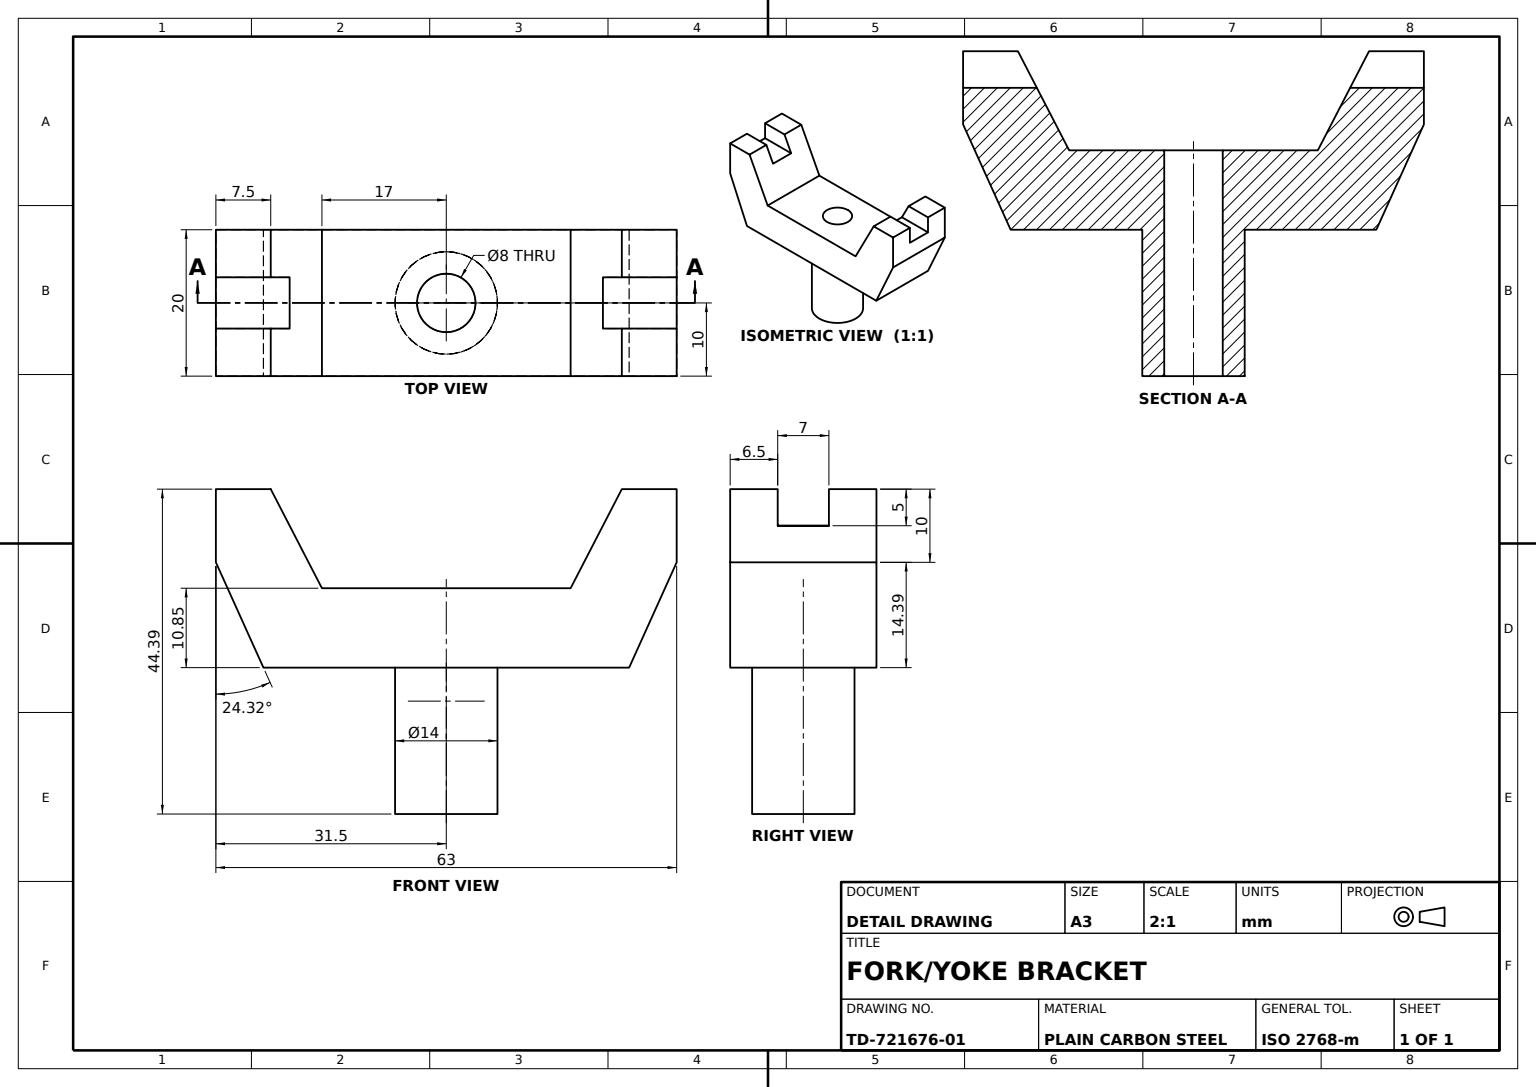
SolidWorks part; units mm, degrees
material "Plain Carbon Steel"
ref_plane "Front Plane" through (0, 0, 0) normal (0, 0, 1) x (1, 0, 0)
ref_plane "Top Plane" through (0, 0, 0) normal (0, 1, 0) x (1, 0, 0)
ref_plane "Right Plane" through (0, 0, 0) normal (1, 0, 0) x (0, 0, -1)
sketch "Yoke Profile Sketch" plane through (0, 0, 0) normal (0, 0, 1) x (1, 0, 0)
  line L0 (0, 0) -> (17, 0)
  line L1 (17, 0) -> (24, 13.5374)
  line L2 (24, 13.5374) -> (31.5, 13.5374)
  line L3 (31.5, 13.5374) -> (31.5, 3.5374)
  line L7 (-31.5, 3.5374) -> (-31.5, 13.5374)
  line L10 (-17, 0) -> (0, 0)
  line L11 (0, 0) -> (0, 32.4855) construction
  line L12 (-17, 0) -> (-24, 13.5374)
  line L13 (-24, 13.5374) -> (-31.5, 13.5374)
  line L17 (0, 0) -> (0, -10.8484) construction
  line L18 (-25, -10.8484) -> (25, -10.8484)
  line L19 (25, -10.8484) -> (31.5, 3.5374)
  line L20 (-25, -10.8484) -> (-31.5, 3.5374)
  dimension "D1" = 10
  dimension "D2" = 17
  dimension "D3" = 6.5
  dimension "D4" = 31.5
  dimension "D5" = 7.5
  dimension "D6" = 10.8484
  dimension "D7" = 14.3858
extrude "Yoke Body" add sketch "Yoke Profile Sketch" along normal mid plane 20
sketch "Arm Slots Sketch" plane through (-31.5, 0, 0) normal (-1, 0, 0) x (0, 0, 1)
  line L0 (0, 13.5374) -> (3.5, 13.5374)
  line L1 (10, 13.5374) -> (-10, 13.5374) construction
  line L2 (3.5, 13.5374) -> (3.5, 8.5374)
  line L3 (3.5, 8.5374) -> (-3.5, 8.5374)
  line L4 (-3.5, 8.5374) -> (-3.5, 13.5374)
  line L5 (-3.5, 13.5374) -> (0, 13.5374)
  line L6 (-10, 13.5374) -> (-10, 3.5374) construction
  line L7 (10, 3.5374) -> (-10, 3.5374) construction
  dimension "D1" = 6.5
  dimension "D2" = 5
extrude "Arm Slots" cut sketch "Arm Slots Sketch" against normal through all
sketch "Post Seat Sketch" plane through (0, 0, 0) normal (0, 1, 0) x (1, 0, 0)
  circle A0 centre (0, 0) radius 4
  dimension "D1" = 8
extrude "Post Seat Cut" cut sketch "Post Seat Sketch" against normal blind 20
sketch "Pivot Post Sketch" plane through (0, -10.8484, 0) normal (0, -1, 0) x (1, 0, 0)
  circle A0 centre (0, 0) radius 7
  dimension "D1" = 14
extrude "Pivot Post" add sketch "Pivot Post Sketch" along normal blind 20
sketch "Centre Hole Sketch" plane through (0, 0, 0) normal (0, 1, 0) x (1, 0, 0)
  circle A0 centre (0, 0) radius 4
  dimension "D1" = 8
extrude "Centre Hole" cut sketch "Centre Hole Sketch" against normal through all
